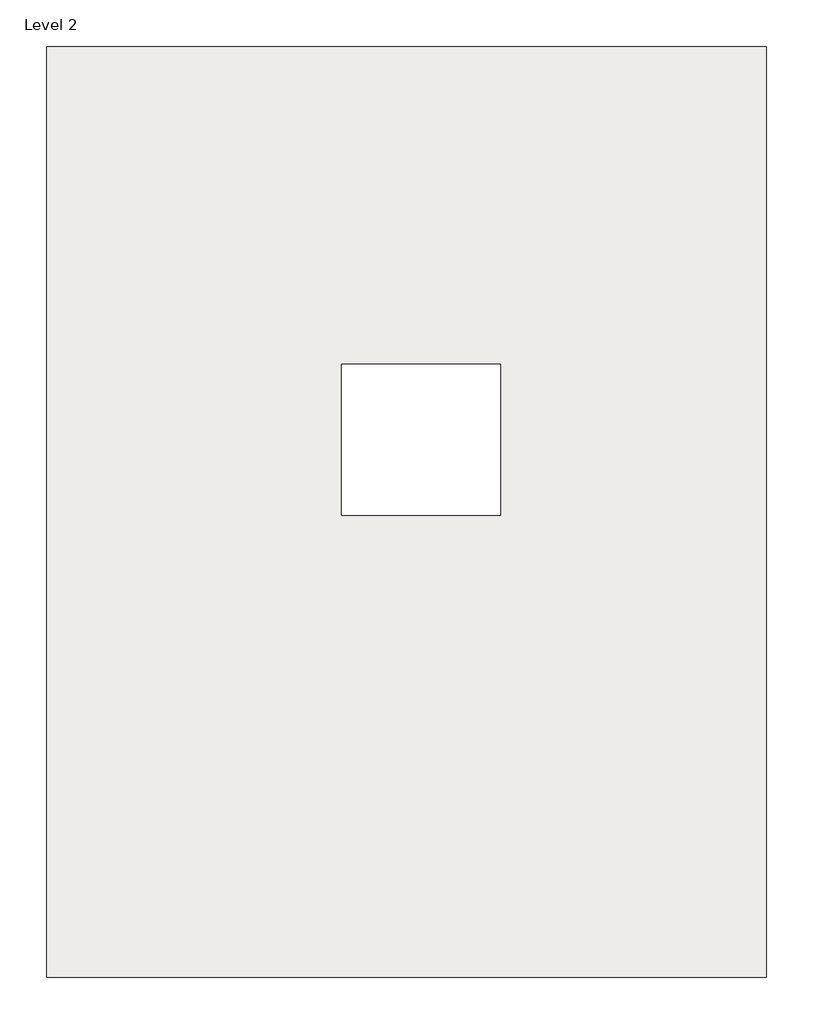
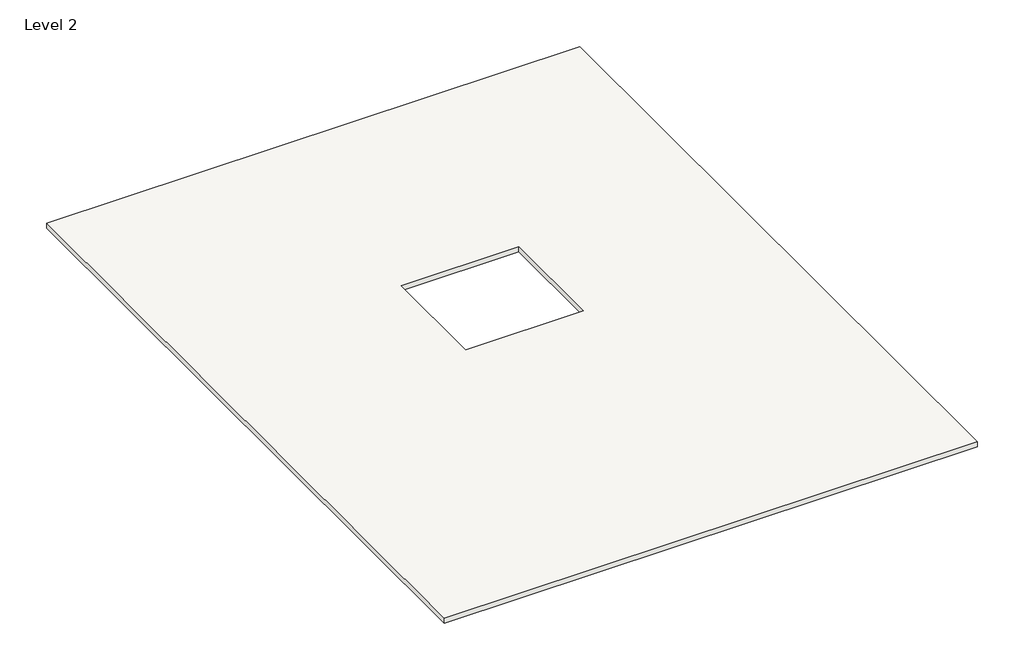
# One storey, incomplete: 1 roof.
"""IFC4 building model written with IfcOpenShell, lengths in millimetres."""

from ifc_helpers import new_model, si_unit, frame, origin, place, context, project, spatial, polyline, outline, extrude, element, save

model = new_model("IFC4")

# Units and contexts
model_context = context("Model", 3, world=origin())
ifc_project = project(units=[si_unit("LENGTHUNIT", "METRE", prefix="MILLI")], contexts=[model_context])

# Site, building, storey
site = spatial("IfcSite", under=ifc_project)
building = spatial("IfcBuilding", under=site)
storey = spatial("IfcBuildingStorey", under=building, Name="Level 2", Elevation=3048.0)

# Roof
placement = place(None, origin())
element("IfcRoof", 1, ObjectType="Generic - 12\"", at=placement, inside=storey, context=model_context, shape_type="SweptSolid", body=[
    extrude(outline(polyline([(-8113.2415084, -8469.6977377), (-8113.2415084, 11037.5022623), (6974.3584916, 11037.5022623), (6974.3584916, -8469.6977377), (-8113.2415084, -8469.6977377)]), holes=[polyline([(1404.6885894, 4375.6877175), (-1922.9455737, 4375.6877175), (-1922.9455737, 1218.1652728), (1404.6885894, 1218.1652728), (1404.6885894, 4375.6877175)])]), frame((0.0, 0.0, 3048.0), z_axis=(0.0, 0.0, 1.0), x_axis=(1.0, 0.0, 0.0)), (0.0, 0.0, 1.0), 152.4),
])

save(model, "model.ifc")

# Revit data of these elements
# Type "Generic - 12\""
#   Assembly Code = "B1020"
#   Layers, outside or top first: 0' - 6" no material (function 1)
# Element 1 (IfcRoof, "Generic - 12\"")
#   built-in parameter 1001705 = 10.5 (stored number, unit not read)
#   built-in parameter 1001710 = 33615
#   Phase Created = New Construction
#   Materials on its faces: "Default Roof", "legs"
# Materials
#   "Default Roof": colour RGB 88 101 114, transparency 0, Cost = 0
#   "legs": colour RGB 90 73 37, transparency 0, Cost = 0
